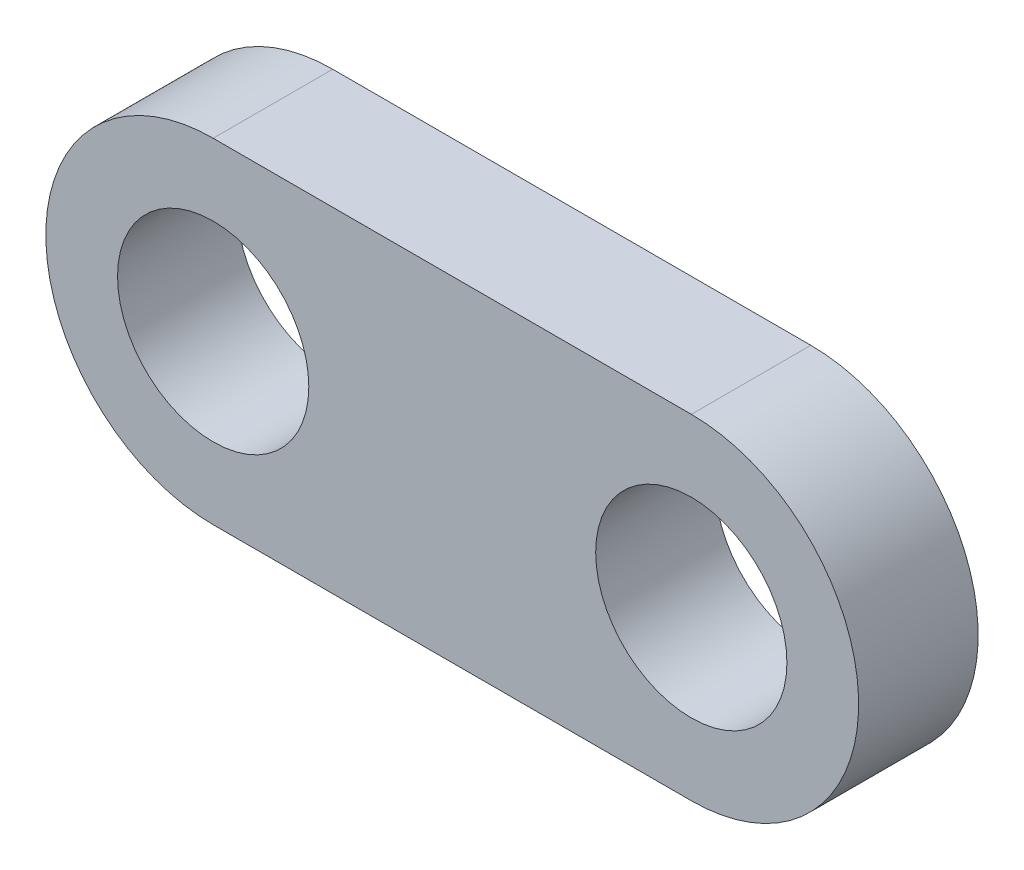
SolidWorks part; units mm, degrees
material "Plain Carbon Steel"
ref_plane "Front Plane" through (0, 0, 0) normal (0, 0, 1) x (1, 0, 0)
ref_plane "Top Plane" through (0, 0, 0) normal (0, 1, 0) x (1, 0, 0)
ref_plane "Right Plane" through (0, 0, 0) normal (1, 0, 0) x (0, 0, -1)
sketch "Link Profile Sketch" plane through (0, 0, 0) normal (0, 0, 1) x (1, 0, 0)
  line L0 (-10, 0) -> (10, 0) construction
  line L1 (-10, 7) -> (10, 7)
  line L2 (-10, -7) -> (10, -7)
  arc A0 (-10, 7) -> (-10, -7) centre (-10, 0) ccw
  arc A1 (10, -7) -> (10, 7) centre (10, 0) ccw
  circle A2 centre (-10, 0) radius 4
  circle A3 centre (10, 0) radius 4
  point P2 (0, 0)
  dimension "D1" = 7
  dimension "D3" = 8
  dimension "D2" = 20
extrude "Link Plate 5mm" add sketch "Link Profile Sketch" along normal mid plane 5
